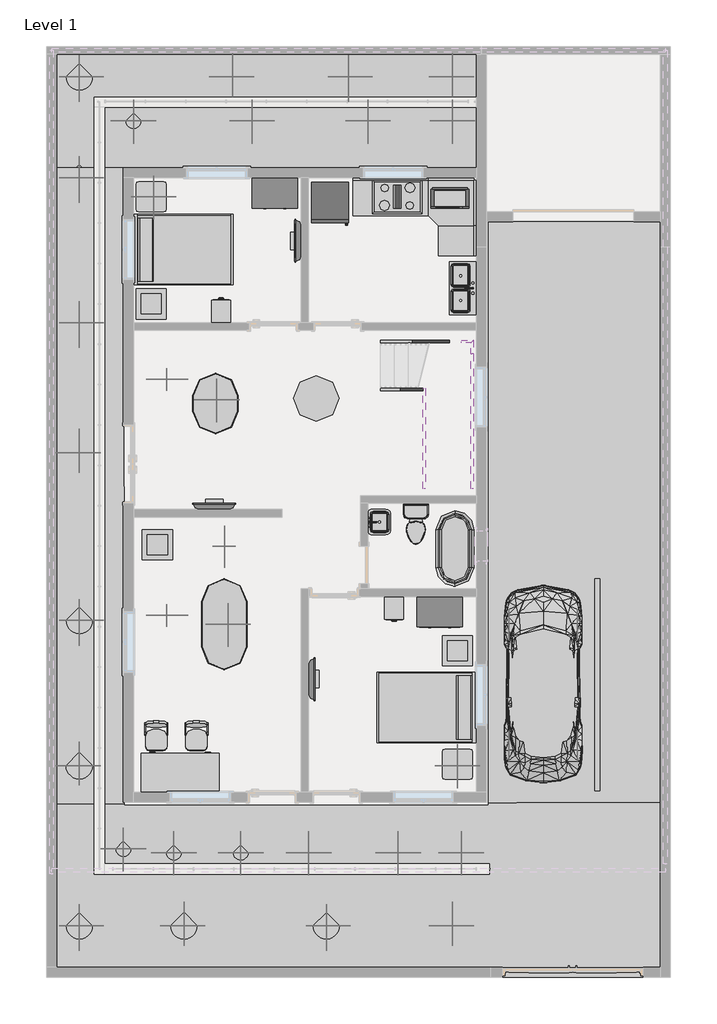
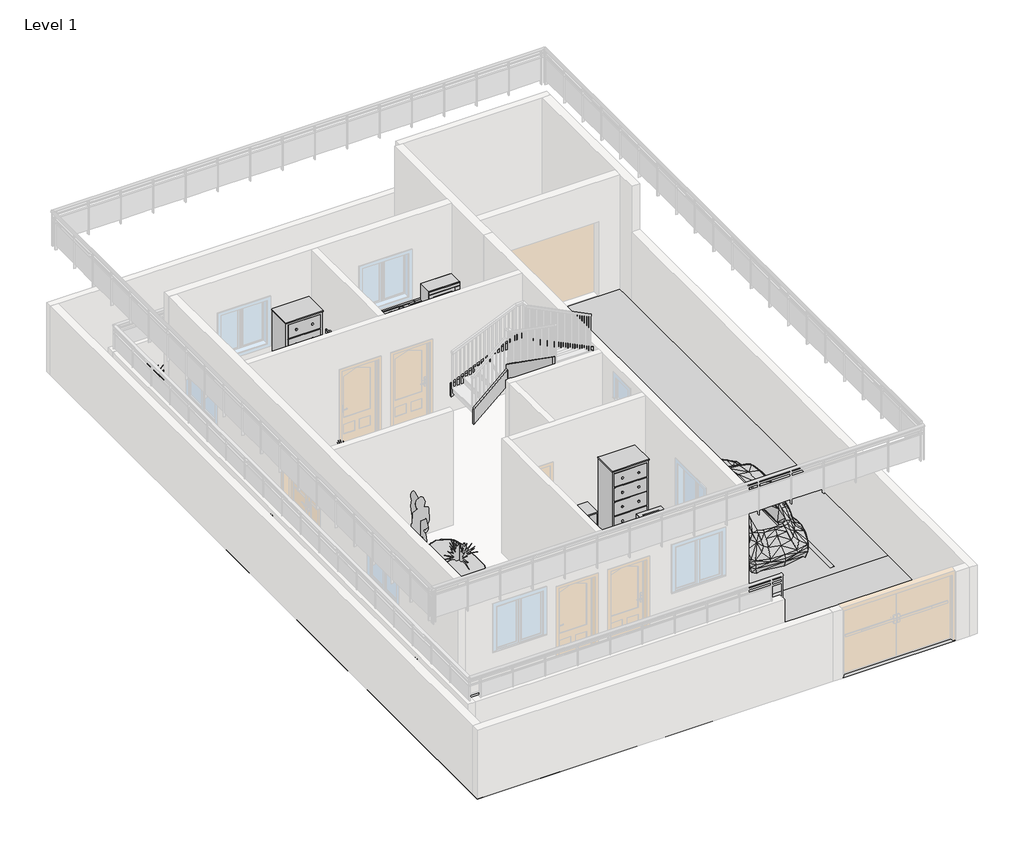
# One storey, part 5 of 5: 27 geographic elements, 21 furniture elements, 12 proxies, 6 members, 5 flow terminals.
"""IFC4 building model written with IfcOpenShell, lengths in millimetres."""

from ifc_helpers import new_model, si_unit, frame, origin, place, context, project, spatial, polyline, outline, extrude, triangles, transform, mapped, element, save
from components import proxy_bb1e6e30, proxy_8a8d5ab2, parking_space_9_x_18_90_deg_fdd9e8f5, rpc_beetle_rpc_beetle_3ce7ba48, rpc_female_69e001fa, proxy_a13a33b2, flow_terminal_accce45a, flow_terminal_a53be723, flow_terminal_62a433f7, toilet_domestic_3d_toilet_domestic_3d_f7549cf7, toilet_domestic_3d_toilet_domestic_3d_183bbd19, flow_terminal_b374fae2, furniture_096e7f55, furniture_bb55ed6b, furniture_072f6425, furniture_33655958, furniture_3d1d9cbc, furniture_56245f3a, furniture_b5c51a22, furniture_be1c6672, furniture_2c34a4f9, furniture_905aceb5, furniture_31d08a24, furniture_4f21b5ed, rpc_plant_tropical_55f6ff97, rpc_plant_tropical_agave_1_5_93a2a214, rpc_plant_tropical_jungle_flame_3_9c4808c2

model = new_model("IFC4")

# Units and contexts
model_context = context("Model", 3, world=origin())
ifc_project = project(units=[si_unit("LENGTHUNIT", "METRE", prefix="MILLI")], contexts=[model_context])

# Site, building, storey
site = spatial("IfcSite", under=ifc_project)
building = spatial("IfcBuilding", under=site)
storey = spatial("IfcBuildingStorey", under=building, Name="Level 1", Elevation=0.0)

# Proxies
placement = place(None, origin())
element("IfcBuildingElementProxy", 1, Name="Building Element Proxy", at=placement, inside=storey, context=model_context, shape_type="Tessellation", body=[
    triangles([(-2362.0350391, 11534.7029114, 0.0), (-2374.735136, 9147.103299, 0.0), (-2273.1350876, 9248.7034927, 0.0), (-11137.7352814, 9245.8391327, 0.0), (-11137.7352814, 11687.1029114, 0.0)], [[5, 4, 1], [2, 3, 1], [2, 1, 4]], closed=False),
])
element("IfcBuildingElementProxy", 2, Name="Building Element Proxy", at=placement, inside=storey, context=model_context, shape_type="Tessellation", body=[
    triangles([(-9588.3350876, 9248.7034927, 0.0), (-11137.7352814, 9247.2006775, 0.0), (-9588.3350876, -3527.4966042, 0.0), (-11137.7352814, -3577.79179, 0.0), (-9562.9348938, -3578.296701, 0.0)], [[2, 4, 3], [3, 5, 1], [5, 3, 4], [3, 1, 2]], closed=False),
])
element("IfcBuildingElementProxy", 3, Name="Building Element Proxy", at=placement, inside=storey, context=model_context, shape_type="Tessellation", body=[
    triangles([(-10934.5348938, -3567.3589966, 0.0), (-11137.7352814, -3577.79179, 0.0), (-11137.7352814, -7058.0965073, 0.0), (1435.264864, -7058.0965073, 0.0), (1435.264864, -3525.6286949, 0.0)], [[2, 3, 1], [1, 4, 5], [4, 1, 3]], closed=False),
])
element("IfcBuildingElementProxy", 4, Name="Building Element Proxy", at=placement, inside=storey, context=model_context, shape_type="Tessellation", body=[
    triangles([(-2273.1350876, -3527.4966042, 0.0), (1435.264864, -3483.8981026, 0.0), (-2273.1350876, 8156.503299, 0.0), (1232.0649124, 8156.503299, 0.0), (1232.0649124, -3528.5849098, 0.0), (-1984.8734676, -3532.3309021, 0.0), (-2247.7350391, -3578.296701, 0.0)], [[6, 3, 1], [6, 1, 7], [6, 5, 4], [5, 6, 7], [2, 4, 5], [6, 4, 3]], closed=False),
])
proxy_shape = proxy_bb1e6e30(model_context)
element("IfcBuildingElementProxy", 5, Name="Cook Top-4 Unit : 36\" x 20\"", ObjectType="Cook Top-4 Unit : 36\" x 20\"", at=placement, inside=storey, context=model_context, shape_type="MappedRepresentation", body=[
    mapped(proxy_shape, transform((-4070.1850785, 8664.5033005, 0.0), x_axis=(1.0, 0.0, 0.0), y_axis=(0.0, 1.0, 0.0), z_axis=(0.0, 0.0, 1.0))),
])
proxy_2_shape = proxy_8a8d5ab2(model_context)
element("IfcBuildingElementProxy", 6, Name="Microwave : 30\" x 16\" x 18\"", ObjectType="Microwave : 30\" x 16\" x 18\"", at=placement, inside=storey, context=model_context, shape_type="MappedRepresentation", body=[
    mapped(proxy_2_shape, transform((-3510.0279559, 8992.1838064, 0.0), x_axis=(1.0, 0.0, 0.0), y_axis=(0.0, 1.0, 0.0), z_axis=(0.0, 0.0, 1.0))),
])
parking_space_9_x_18_90_deg_shape = parking_space_9_x_18_90_deg_fdd9e8f5(model_context)
element("IfcBuildingElementProxy", 7, Name="Parking Space : 9' x 18' - 90 deg", ObjectType="Parking Space : 9' x 18' - 90 deg", at=placement, inside=storey, context=model_context, shape_type="MappedRepresentation", body=[
    mapped(parking_space_9_x_18_90_deg_shape, transform((-37.9350785, -3298.8966995, 0.0), x_axis=(-1.0000000000000004, 0.0, 0.0), y_axis=(0.0, -1.0000000000000004, 0.0), z_axis=(0.0, 0.0, 1.0))),
])
rpc_beetle_rpc_beetle_shape = rpc_beetle_rpc_beetle_3ce7ba48(model_context)
element("IfcBuildingElementProxy", 8, Name="RPC Beetle : RPC Beetle", ObjectType="RPC Beetle : RPC Beetle", at=placement, inside=storey, context=model_context, shape_type="MappedRepresentation", body=[
    mapped(rpc_beetle_rpc_beetle_shape, transform((-1130.1350785, -2384.4966995, 0.0), x_axis=(1.0, 0.0, 0.0), y_axis=(0.0, 1.0, 0.0), z_axis=(0.0, 0.0, 1.0))),
])
rpc_female_shape = rpc_female_69e001fa(model_context)
element("IfcBuildingElementProxy", 9, Name="RPC Female", ObjectType="RPC Female", at=placement, inside=storey, context=model_context, shape_type="MappedRepresentation", body=[
    mapped(rpc_female_shape, transform((-7557.9773474, 1463.6033005, 0.0), x_axis=(1.0, 0.0, 0.0), y_axis=(0.0, 1.0, 0.0), z_axis=(0.0, 0.0, 1.0))),
])
element("IfcBuildingElementProxy", 10, Name="RPC Female", ObjectType="RPC Female", at=placement, inside=storey, context=model_context, shape_type="MappedRepresentation", body=[
    mapped(rpc_female_shape, transform((-8559.6350785, 231.7033005, 0.0), x_axis=(0.0, 1.0, 0.0), y_axis=(-1.0, 0.0, 0.0), z_axis=(0.0, 0.0, 1.0))),
])
element("IfcBuildingElementProxy", 11, Name="RPC Female", ObjectType="RPC Female", at=placement, inside=storey, context=model_context, shape_type="MappedRepresentation", body=[
    mapped(rpc_female_shape, transform((-8559.6350785, 4981.5033005, 0.0), x_axis=(0.0, 1.0, 0.0), y_axis=(-1.0, 0.0, 0.0), z_axis=(0.0, 0.0, 1.0))),
])
proxy_3_shape = proxy_a13a33b2(model_context)
element("IfcBuildingElementProxy", 12, Name="Refrigerator : 30\" x 32\" RH", ObjectType="Refrigerator : 30\" x 32\" RH", at=placement, inside=storey, context=model_context, shape_type="MappedRepresentation", body=[
    mapped(proxy_3_shape, transform((-5427.4975785, 8561.704329, 0.0), x_axis=(1.0, 0.0, 0.0), y_axis=(0.0, 1.0, 0.0), z_axis=(0.0, 0.0, 1.0))),
])

# Flow terminals
flow_terminal_shape = flow_terminal_accce45a(model_context)
element("IfcFlowTerminal", 13, ObjectType="Floor Drain - Round : 5\" Strainer - 2\" Drain", at=placement, inside=storey, context=model_context, shape_type="MappedRepresentation", body=[
    mapped(flow_terminal_shape, transform((-3492.3350785, 942.9033005, 0.0), x_axis=(1.0, 0.0, 0.0), y_axis=(0.0, 1.0, 0.0), z_axis=(0.0, 0.0, 1.0))),
])
flow_terminal_2_shape = flow_terminal_a53be723(model_context)
element("IfcFlowTerminal", 14, ObjectType="Sink Kitchen-Double : 42\" x 21\"", at=placement, inside=storey, context=model_context, shape_type="MappedRepresentation", body=[
    mapped(flow_terminal_2_shape, transform((-2758.0804796, 6838.6925411, 0.0), x_axis=(0.0, -1.0000000000000004, 0.0), y_axis=(1.0000000000000004, 0.0, 0.0), z_axis=(0.0, 0.0, 1.0))),
])
flow_terminal_3_shape = flow_terminal_62a433f7(model_context)
element("IfcFlowTerminal", 15, ObjectType="Sink Vanity-Square : 20\" x 18\"", at=placement, inside=storey, context=model_context, shape_type="MappedRepresentation", body=[
    mapped(flow_terminal_3_shape, transform((-4480.5896774, 2095.61406, 0.0), x_axis=(0.0, 1.0000000000000002, 0.0), y_axis=(-1.0000000000000002, 0.0, 0.0), z_axis=(0.0, 0.0, 1.0))),
])
toilet_domestic_3d_toilet_domestic_3d_shape = toilet_domestic_3d_toilet_domestic_3d_f7549cf7(model_context)
toilet_domestic_3d_toilet_domestic_3d_2_shape = toilet_domestic_3d_toilet_domestic_3d_183bbd19(model_context)
element("IfcFlowTerminal", 16, ObjectType="Toilet-Domestic-3D : Toilet-Domestic-3D", at=placement, inside=storey, context=model_context, shape_type="MappedRepresentation", body=[
    mapped(toilet_domestic_3d_toilet_domestic_3d_shape, transform((-3695.5350785, 1972.2072732, 0.0), x_axis=(1.0, 0.0, 0.0), y_axis=(0.0, 1.0, 0.0), z_axis=(0.0, 0.0, 1.0))),
    mapped(toilet_domestic_3d_toilet_domestic_3d_2_shape, transform((-3695.5350785, 1972.2072732, 0.0), x_axis=(1.0, 0.0, 0.0), y_axis=(0.0, 1.0, 0.0), z_axis=(0.0, 0.0, 1.0))),
])
flow_terminal_4_shape = flow_terminal_b374fae2(model_context)
element("IfcFlowTerminal", 17, ObjectType="Tub-Free Standing-3D : 30\" x 60\"", at=placement, inside=storey, context=model_context, shape_type="MappedRepresentation", body=[
    mapped(flow_terminal_4_shape, transform((-2908.1350785, 1577.9033005, 0.0), x_axis=(1.0, 0.0, 0.0), y_axis=(0.0, 1.0, 0.0), z_axis=(0.0, 0.0, 1.0))),
])

# Furniture
furniture_shape = furniture_096e7f55(model_context)
element("IfcFurniture", 18, ObjectType="Bed-Shaker : Double 56\" x 78\"", at=placement, inside=storey, context=model_context, shape_type="MappedRepresentation", body=[
    mapped(furniture_shape, transform((-9359.7350785, 7616.7533005, 0.0), x_axis=(0.0, 1.0000000000000002, 0.0), y_axis=(-1.0000000000000002, 0.0, 0.0), z_axis=(0.0, 0.0, 1.0))),
])
element("IfcFurniture", 19, ObjectType="Bed-Shaker : Double 56\" x 78\"", at=placement, inside=storey, context=model_context, shape_type="MappedRepresentation", body=[
    mapped(furniture_shape, transform((-2501.7350785, -1641.5466995, 0.0), x_axis=(0.0, -1.0000000000000002, 0.0), y_axis=(1.0000000000000002, 0.0, 0.0), z_axis=(0.0, 0.0, 1.0))),
])
furniture_2_shape = furniture_bb55ed6b(model_context)
element("IfcFurniture", 20, ObjectType="Cabinet-File 2 Drawer : 15\" x 18\"", at=placement, inside=storey, context=model_context, shape_type="MappedRepresentation", body=[
    mapped(furniture_2_shape, transform((-7747.7315256, 6210.9690004, 0.0), x_axis=(-1.0, 0.0, 0.0), y_axis=(0.0, -1.0, 0.0), z_axis=(0.0, 0.0, 1.0))),
])
element("IfcFurniture", 21, ObjectType="Cabinet-File 2 Drawer : 15\" x 18\"", at=placement, inside=storey, context=model_context, shape_type="MappedRepresentation", body=[
    mapped(furniture_2_shape, transform((-4004.9552228, 526.2376007, 0.0), x_axis=(1.0, 0.0, 0.0), y_axis=(0.0, 1.0, 0.0), z_axis=(0.0, 0.0, 1.0))),
])
furniture_3_shape = furniture_072f6425(model_context)
element("IfcFurniture", 22, ObjectType="Desk : 60\" x 30\" Student", at=placement, inside=storey, context=model_context, shape_type="MappedRepresentation", body=[
    mapped(furniture_3_shape, transform((-9207.3350785, -3324.2966995, 0.0), x_axis=(1.0, 0.0, 0.0), y_axis=(0.0, 1.0, 0.0), z_axis=(0.0, 0.0, 1.0))),
])
furniture_4_shape = furniture_33655958(model_context)
element("IfcFurniture", 23, ObjectType="Dresser : 48\" x 72\" x 24\"", at=placement, inside=storey, context=model_context, shape_type="MappedRepresentation", body=[
    mapped(furniture_4_shape, transform((-6271.1418187, 9103.8662546, 0.0), x_axis=(1.0, 0.0, 0.0), y_axis=(0.0, 1.0, 0.0), z_axis=(0.0, 0.0, 1.0))),
])
element("IfcFurniture", 24, ObjectType="Dresser : 48\" x 72\" x 24\"", at=placement, inside=storey, context=model_context, shape_type="MappedRepresentation", body=[
    mapped(furniture_4_shape, transform((-2943.7418187, 671.0662546, 0.0), x_axis=(1.0, 0.0, 0.0), y_axis=(0.0, 1.0, 0.0), z_axis=(0.0, 0.0, 1.0))),
])
furniture_5_shape = furniture_3d1d9cbc(model_context)
element("IfcFurniture", 25, ObjectType="Seating-Auditorium : 18\" x 24\" x 30\"", at=placement, inside=storey, context=model_context, shape_type="MappedRepresentation", body=[
    mapped(furniture_5_shape, transform((-8767.2072097, -1991.4212896, 0.0), x_axis=(-1.0000000000000004, 0.0, 0.0), y_axis=(0.0, -1.0000000000000004, 0.0), z_axis=(0.0, 0.0, 1.0))),
])
element("IfcFurniture", 26, ObjectType="Seating-Auditorium : 18\" x 24\" x 30\"", at=placement, inside=storey, context=model_context, shape_type="MappedRepresentation", body=[
    mapped(furniture_5_shape, transform((-7954.4072097, -1991.4212896, 0.0), x_axis=(-1.0, 0.0, 0.0), y_axis=(0.0, -1.0, 0.0), z_axis=(0.0, 0.0, 1.0))),
])
furniture_6_shape = furniture_56245f3a(model_context)
element("IfcFurniture", 27, ObjectType="TV - Flat Screen : 32\"", at=placement, inside=storey, context=model_context, shape_type="MappedRepresentation", body=[
    mapped(furniture_6_shape, transform((-6065.4737022, 7771.5587864, 914.4), x_axis=(0.0, -1.0000000000000004, 0.0), y_axis=(1.0000000000000004, 0.0, 0.0), z_axis=(0.0, 0.0, 1.0))),
])
element("IfcFurniture", 28, ObjectType="TV - Flat Screen : 32\"", at=placement, inside=storey, context=model_context, shape_type="MappedRepresentation", body=[
    mapped(furniture_6_shape, transform((-7763.4795927, 2423.8419242, 1041.4), x_axis=(-1.0, 0.0, 0.0), y_axis=(0.0, -1.0, 0.0), z_axis=(0.0, 0.0, 1.0))),
])
element("IfcFurniture", 29, ObjectType="TV - Flat Screen : 32\"", at=placement, inside=storey, context=model_context, shape_type="MappedRepresentation", body=[
    mapped(furniture_6_shape, transform((-5795.9964549, -1047.0521853, 1041.4), x_axis=(0.0, 1.0000000000000002, 0.0), y_axis=(-1.0000000000000002, 0.0, 0.0), z_axis=(0.0, 0.0, 1.0))),
])
furniture_7_shape = furniture_b5c51a22(model_context)
element("IfcFurniture", 30, ObjectType="Table-Coffee : 24\" x 24\" x 24\"", at=placement, inside=storey, context=model_context, shape_type="MappedRepresentation", body=[
    mapped(furniture_7_shape, transform((-9047.8008452, 6410.2922227, 0.0), x_axis=(1.0, 0.0, 0.0), y_axis=(0.0, 1.0, 0.0), z_axis=(0.0, 0.0, 1.0))),
])
element("IfcFurniture", 31, ObjectType="Table-Coffee : 24\" x 24\" x 24\"", at=placement, inside=storey, context=model_context, shape_type="MappedRepresentation", body=[
    mapped(furniture_7_shape, transform((-2875.6008452, -574.7077773, 0.0), x_axis=(1.0, 0.0, 0.0), y_axis=(0.0, 1.0, 0.0), z_axis=(0.0, 0.0, 1.0))),
])
element("IfcFurniture", 32, ObjectType="Table-Coffee : 24\" x 24\" x 24\"", at=placement, inside=storey, context=model_context, shape_type="MappedRepresentation", body=[
    mapped(furniture_7_shape, transform((-8920.8008452, 1558.8922227, 0.0), x_axis=(1.0, 0.0, 0.0), y_axis=(0.0, 1.0, 0.0), z_axis=(0.0, 0.0, 1.0))),
])
furniture_8_shape = furniture_be1c6672(model_context)
element("IfcFurniture", 33, ObjectType="Table-Dining Oval : 36\" x 48\"", at=placement, inside=storey, context=model_context, shape_type="MappedRepresentation", body=[
    mapped(furniture_8_shape, transform((-8092.2334392, 4900.7229727, 0.0), x_axis=(0.0, 1.0000000000000002, 0.0), y_axis=(-1.0000000000000002, 0.0, 0.0), z_axis=(0.0, 0.0, 1.0))),
])
furniture_9_shape = furniture_2c34a4f9(model_context)
element("IfcFurniture", 34, ObjectType="Table-Dining Oval : 36\" x 72\"", at=placement, inside=storey, context=model_context, shape_type="MappedRepresentation", body=[
    mapped(furniture_9_shape, transform((-7914.4334392, 455.7229727, 0.0), x_axis=(0.0, 1.0, 0.0), y_axis=(-1.0, 0.0, 0.0), z_axis=(0.0, 0.0, 1.0))),
])
furniture_10_shape = furniture_905aceb5(model_context)
element("IfcFurniture", 35, ObjectType="Table-Dining Round w Chairs : 36\" Diameter", at=placement, inside=storey, context=model_context, shape_type="MappedRepresentation", body=[
    mapped(furniture_10_shape, transform((-5805.8170457, 4785.3819891, 0.0), x_axis=(1.0, 0.0, 0.0), y_axis=(0.0, 1.0, 0.0), z_axis=(0.0, 0.0, 1.0))),
])
furniture_11_shape = furniture_31d08a24(model_context)
element("IfcFurniture", 36, ObjectType="Table-End : 24\" x 24\"", at=placement, inside=storey, context=model_context, shape_type="MappedRepresentation", body=[
    mapped(furniture_11_shape, transform((-9338.0687088, 8512.1033005, 0.0), x_axis=(1.0, 0.0, 0.0), y_axis=(0.0, 1.0, 0.0), z_axis=(0.0, 0.0, 1.0))),
])
element("IfcFurniture", 37, ObjectType="Table-End : 24\" x 24\"", at=placement, inside=storey, context=model_context, shape_type="MappedRepresentation", body=[
    mapped(furniture_11_shape, transform((-3165.8687088, -2917.8966995, 0.0), x_axis=(1.0, 0.0, 0.0), y_axis=(0.0, 1.0, 0.0), z_axis=(0.0, 0.0, 1.0))),
])
furniture_12_shape = furniture_4f21b5ed(model_context)
element("IfcFurniture", 38, ObjectType="Work Station Cubicle : 96\" x 96\"", at=placement, inside=storey, context=model_context, shape_type="MappedRepresentation", body=[
    mapped(furniture_12_shape, transform((-1981.3120709, 8913.7715483, 0.0), x_axis=(0.0, -0.9999999999999998, 0.0), y_axis=(0.9999999999999998, 0.0, 0.0), z_axis=(0.0, 0.0, 1.0))),
])

# Geographic elements
rpc_plant_tropical_shape = rpc_plant_tropical_55f6ff97(model_context)
element("IfcGeographicElement", 39, ObjectType="RPC Plant - Tropical", at=placement, inside=storey, context=model_context, shape_type="MappedRepresentation", body=[
    mapped(rpc_plant_tropical_shape, transform((-5054.4350785, 11077.5033005, 0.0), x_axis=(1.0, 0.0, 0.0), y_axis=(0.0, 1.0, 0.0), z_axis=(0.0, 0.0, 1.0))),
])
element("IfcGeographicElement", 40, ObjectType="RPC Plant - Tropical", at=placement, inside=storey, context=model_context, shape_type="MappedRepresentation", body=[
    mapped(rpc_plant_tropical_shape, transform((-10477.3350785, 11077.5033005, 0.0), x_axis=(1.0, 0.0, 0.0), y_axis=(0.0, 1.0, 0.0), z_axis=(0.0, 0.0, 1.0))),
])
element("IfcGeographicElement", 41, ObjectType="RPC Plant - Tropical", at=placement, inside=storey, context=model_context, shape_type="MappedRepresentation", body=[
    mapped(rpc_plant_tropical_shape, transform((-10477.3350785, 9045.5033005, 0.0), x_axis=(1.0, 0.0, 0.0), y_axis=(0.0, 1.0, 0.0), z_axis=(0.0, 0.0, 1.0))),
])
element("IfcGeographicElement", 42, ObjectType="RPC Plant - Tropical", at=placement, inside=storey, context=model_context, shape_type="MappedRepresentation", body=[
    mapped(rpc_plant_tropical_shape, transform((-10477.3350785, 6124.5033005, 0.0), x_axis=(1.0, 0.0, 0.0), y_axis=(0.0, 1.0, 0.0), z_axis=(0.0, 0.0, 1.0))),
])
element("IfcGeographicElement", 43, ObjectType="RPC Plant - Tropical", at=placement, inside=storey, context=model_context, shape_type="MappedRepresentation", body=[
    mapped(rpc_plant_tropical_shape, transform((-10477.3350785, 130.1033005, 0.0), x_axis=(1.0, 0.0, 0.0), y_axis=(0.0, 1.0, 0.0), z_axis=(0.0, 0.0, 1.0))),
])
element("IfcGeographicElement", 44, ObjectType="RPC Plant - Tropical", at=placement, inside=storey, context=model_context, shape_type="MappedRepresentation", body=[
    mapped(rpc_plant_tropical_shape, transform((-10477.3350785, -6016.6966995, 0.0), x_axis=(1.0, 0.0, 0.0), y_axis=(0.0, 1.0, 0.0), z_axis=(0.0, 0.0, 1.0))),
])
element("IfcGeographicElement", 45, ObjectType="RPC Plant - Tropical", at=placement, inside=storey, context=model_context, shape_type="MappedRepresentation", body=[
    mapped(rpc_plant_tropical_shape, transform((-5498.9350785, -6016.6966995, 0.0), x_axis=(1.0, 0.0, 0.0), y_axis=(0.0, 1.0, 0.0), z_axis=(0.0, 0.0, 1.0))),
])
rpc_plant_tropical_agave_1_5_shape = rpc_plant_tropical_agave_1_5_93a2a214(model_context)
element("IfcGeographicElement", 46, ObjectType="RPC Plant - Tropical : Agave - 1.5'", at=placement, inside=storey, context=model_context, shape_type="MappedRepresentation", body=[
    mapped(rpc_plant_tropical_agave_1_5_shape, transform((-2958.9350785, 10188.5033005, 0.0), x_axis=(1.0, 0.0, 0.0), y_axis=(0.0, 1.0, 0.0), z_axis=(0.0, 0.0, 1.0))),
])
element("IfcGeographicElement", 47, ObjectType="RPC Plant - Tropical : Agave - 1.5'", at=placement, inside=storey, context=model_context, shape_type="MappedRepresentation", body=[
    mapped(rpc_plant_tropical_agave_1_5_shape, transform((-4660.7350785, 10188.5033005, 0.0), x_axis=(1.0, 0.0, 0.0), y_axis=(0.0, 1.0, 0.0), z_axis=(0.0, 0.0, 1.0))),
])
element("IfcGeographicElement", 48, ObjectType="RPC Plant - Tropical : Agave - 1.5'", at=placement, inside=storey, context=model_context, shape_type="MappedRepresentation", body=[
    mapped(rpc_plant_tropical_agave_1_5_shape, transform((-6997.5350785, 10188.5033005, 0.0), x_axis=(1.0, 0.0, 0.0), y_axis=(0.0, 1.0, 0.0), z_axis=(0.0, 0.0, 1.0))),
])
element("IfcGeographicElement", 49, ObjectType="RPC Plant - Tropical : Agave - 1.5'", at=placement, inside=storey, context=model_context, shape_type="MappedRepresentation", body=[
    mapped(rpc_plant_tropical_agave_1_5_shape, transform((-9385.1350785, 10188.5033005, 0.0), x_axis=(1.0, 0.0, 0.0), y_axis=(0.0, 1.0, 0.0), z_axis=(0.0, 0.0, 1.0))),
])
element("IfcGeographicElement", 50, ObjectType="RPC Plant - Tropical : Agave - 1.5'", at=placement, inside=storey, context=model_context, shape_type="MappedRepresentation", body=[
    mapped(rpc_plant_tropical_agave_1_5_shape, transform((-2781.1350785, -4543.4966995, 0.0), x_axis=(1.0, 0.0, 0.0), y_axis=(0.0, 1.0, 0.0), z_axis=(0.0, 0.0, 1.0))),
])
element("IfcGeographicElement", 51, ObjectType="RPC Plant - Tropical : Agave - 1.5'", at=placement, inside=storey, context=model_context, shape_type="MappedRepresentation", body=[
    mapped(rpc_plant_tropical_agave_1_5_shape, transform((-9588.3350785, -4467.2966995, 0.0), x_axis=(1.0, 0.0, 0.0), y_axis=(0.0, 1.0, 0.0), z_axis=(0.0, 0.0, 1.0))),
])
element("IfcGeographicElement", 52, ObjectType="RPC Plant - Tropical : Agave - 1.5'", at=placement, inside=storey, context=model_context, shape_type="MappedRepresentation", body=[
    mapped(rpc_plant_tropical_agave_1_5_shape, transform((-8572.3350785, -4543.4966995, 0.0), x_axis=(1.0, 0.0, 0.0), y_axis=(0.0, 1.0, 0.0), z_axis=(0.0, 0.0, 1.0))),
])
element("IfcGeographicElement", 53, ObjectType="RPC Plant - Tropical : Agave - 1.5'", at=placement, inside=storey, context=model_context, shape_type="MappedRepresentation", body=[
    mapped(rpc_plant_tropical_agave_1_5_shape, transform((-7226.1350785, -4543.4966995, 0.0), x_axis=(1.0, 0.0, 0.0), y_axis=(0.0, 1.0, 0.0), z_axis=(0.0, 0.0, 1.0))),
])
element("IfcGeographicElement", 54, ObjectType="RPC Plant - Tropical : Agave - 1.5'", at=placement, inside=storey, context=model_context, shape_type="MappedRepresentation", body=[
    mapped(rpc_plant_tropical_agave_1_5_shape, transform((-5854.5350785, -4543.4966995, 0.0), x_axis=(1.0, 0.0, 0.0), y_axis=(0.0, 1.0, 0.0), z_axis=(0.0, 0.0, 1.0))),
])
element("IfcGeographicElement", 55, ObjectType="RPC Plant - Tropical : Agave - 1.5'", at=placement, inside=storey, context=model_context, shape_type="MappedRepresentation", body=[
    mapped(rpc_plant_tropical_agave_1_5_shape, transform((-4051.1350785, -4543.4966995, 0.0), x_axis=(1.0, 0.0, 0.0), y_axis=(0.0, 1.0, 0.0), z_axis=(0.0, 0.0, 1.0))),
])
element("IfcGeographicElement", 56, ObjectType="RPC Plant - Tropical : Agave - 1.5'", at=placement, inside=storey, context=model_context, shape_type="MappedRepresentation", body=[
    mapped(rpc_plant_tropical_agave_1_5_shape, transform((-8978.7350785, 8664.5033005, 609.6), x_axis=(1.0, 0.0, 0.0), y_axis=(0.0, 1.0, 0.0), z_axis=(0.0, 0.0, 1.0))),
])
element("IfcGeographicElement", 57, ObjectType="RPC Plant - Tropical : Agave - 1.5'", at=placement, inside=storey, context=model_context, shape_type="MappedRepresentation", body=[
    mapped(rpc_plant_tropical_agave_1_5_shape, transform((-7708.7350785, 4575.1033005, 736.6), x_axis=(1.0, 0.0, 0.0), y_axis=(0.0, 1.0, 0.0), z_axis=(0.0, 0.0, 1.0))),
])
element("IfcGeographicElement", 58, ObjectType="RPC Plant - Tropical : Agave - 1.5'", at=placement, inside=storey, context=model_context, shape_type="MappedRepresentation", body=[
    mapped(rpc_plant_tropical_agave_1_5_shape, transform((-2857.3350785, -2790.8966995, 609.6), x_axis=(1.0, 0.0, 0.0), y_axis=(0.0, 1.0, 0.0), z_axis=(0.0, 0.0, 1.0))),
])
element("IfcGeographicElement", 59, ObjectType="RPC Plant - Tropical : Agave - 1.5'", at=placement, inside=storey, context=model_context, shape_type="MappedRepresentation", body=[
    mapped(rpc_plant_tropical_agave_1_5_shape, transform((-7480.1350785, 53.9033005, 736.6), x_axis=(1.0, 0.0, 0.0), y_axis=(0.0, 1.0, 0.0), z_axis=(0.0, 0.0, 1.0))),
])
rpc_plant_tropical_jungle_flame_3_shape = rpc_plant_tropical_jungle_flame_3_9c4808c2(model_context)
element("IfcGeographicElement", 60, ObjectType="RPC Plant - Tropical : Jungle Flame - 3'", at=placement, inside=storey, context=model_context, shape_type="MappedRepresentation", body=[
    mapped(rpc_plant_tropical_jungle_flame_3_shape, transform((-2958.9350785, 11077.5033005, 0.0), x_axis=(1.0, 0.0, 0.0), y_axis=(0.0, 1.0, 0.0), z_axis=(0.0, 0.0, 1.0))),
])
element("IfcGeographicElement", 61, ObjectType="RPC Plant - Tropical : Jungle Flame - 3'", at=placement, inside=storey, context=model_context, shape_type="MappedRepresentation", body=[
    mapped(rpc_plant_tropical_jungle_flame_3_shape, transform((-7391.2350785, 11077.5033005, 0.0), x_axis=(1.0, 0.0, 0.0), y_axis=(0.0, 1.0, 0.0), z_axis=(0.0, 0.0, 1.0))),
])
element("IfcGeographicElement", 62, ObjectType="RPC Plant - Tropical : Jungle Flame - 3'", at=placement, inside=storey, context=model_context, shape_type="MappedRepresentation", body=[
    mapped(rpc_plant_tropical_jungle_flame_3_shape, transform((-10477.3350785, 3508.3033005, 0.0), x_axis=(1.0, 0.0, 0.0), y_axis=(0.0, 1.0, 0.0), z_axis=(0.0, 0.0, 1.0))),
])
element("IfcGeographicElement", 63, ObjectType="RPC Plant - Tropical : Jungle Flame - 3'", at=placement, inside=storey, context=model_context, shape_type="MappedRepresentation", body=[
    mapped(rpc_plant_tropical_jungle_flame_3_shape, transform((-10477.3350785, -2790.8966995, 0.0), x_axis=(1.0, 0.0, 0.0), y_axis=(0.0, 1.0, 0.0), z_axis=(0.0, 0.0, 1.0))),
])
element("IfcGeographicElement", 64, ObjectType="RPC Plant - Tropical : Jungle Flame - 3'", at=placement, inside=storey, context=model_context, shape_type="MappedRepresentation", body=[
    mapped(rpc_plant_tropical_jungle_flame_3_shape, transform((-8369.1350785, -6016.6966995, 0.0), x_axis=(1.0, 0.0, 0.0), y_axis=(0.0, 1.0, 0.0), z_axis=(0.0, 0.0, 1.0))),
])
element("IfcGeographicElement", 65, ObjectType="RPC Plant - Tropical : Jungle Flame - 3'", at=placement, inside=storey, context=model_context, shape_type="MappedRepresentation", body=[
    mapped(rpc_plant_tropical_jungle_flame_3_shape, transform((-2958.9350785, -6016.6966995, 0.0), x_axis=(1.0, 0.0, 0.0), y_axis=(0.0, 1.0, 0.0), z_axis=(0.0, 0.0, 1.0))),
])

# Members
element("IfcMember", 66, ObjectType="Stringer - 2\" Width", at=placement, inside=storey, context=model_context, shape_type="SweptSolid", body=[
    extrude(outline(polyline([(922.8849999, -4406.7350785), (590.0562463, -4406.7350785), (1305.2683876, -2776.0728858), (1638.0971411, -2776.0728858), (922.8849999, -4406.7350785)])), frame((0.0, 5718.1033005, 0.0), z_axis=(0.0, 1.0, 0.0), x_axis=(0.0, 0.0, 1.0)), (0.0, 0.0, 1.0), 50.8),
])
element("IfcMember", 67, ObjectType="Stringer - 2\" Width", at=placement, inside=storey, context=model_context, shape_type="SweptSolid", body=[
    extrude(outline(polyline([(-2776.0728858, 5718.1033005), (-2776.0728858, 5768.9033005), (-2537.598089, 5768.9033005), (-2588.398089, 5718.1033005), (-2776.0728858, 5718.1033005)])), frame((0.0, 0.0, 1305.2683876), z_axis=(0.0, 0.0, 1.0), x_axis=(1.0, 0.0, 0.0)), (0.0, 0.0, 1.0), 332.8287535),
])
element("IfcMember", 68, ObjectType="Stringer - 2\" Width", at=placement, inside=storey, context=model_context, shape_type="SweptSolid", body=[
    extrude(outline(polyline([(-2588.398089, 5718.1033005), (-2537.598089, 5768.9033005), (-2537.598089, 5499.9499575), (-2588.398089, 5499.9499575), (-2588.398089, 5718.1033005)])), frame((0.0, 0.0, 1305.2683876), z_axis=(0.0, 0.0, 1.0), x_axis=(1.0, 0.0, 0.0)), (0.0, 0.0, 1.0), 332.8287535),
])
element("IfcMember", 69, ObjectType="Stringer - 2\" Width", at=placement, inside=storey, context=model_context, shape_type="SweptSolid", body=[
    extrude(outline(polyline([(5499.9499575, 1638.0971411), (5499.9499575, 1305.2683876), (2782.166311, 2720.7901969), (2782.166311, 3053.6189504), (5499.9499575, 1638.0971411)])), frame((-2588.398089, 0.0, 0.0), z_axis=(1.0, 0.0, 0.0), x_axis=(0.0, 1.0, 0.0)), (0.0, 0.0, 1.0), 50.8),
])
element("IfcMember", 70, ObjectType="Stringer - 2\" Width", at=placement, inside=storey, context=model_context, shape_type="SweptSolid", body=[
    extrude(outline(polyline([(842.634734, -4406.7350785), (435.4922729, -4406.7350785), (1191.0265733, -3553.598089), (1598.1690344, -3553.598089), (842.634734, -4406.7350785)])), frame((0.0, 4752.9033005, 0.0), z_axis=(0.0, 1.0, 0.0), x_axis=(0.0, 0.0, 1.0)), (0.0, 0.0, 1.0), 50.8),
])
element("IfcMember", 71, ObjectType="Stringer - 2\" Width", at=placement, inside=storey, context=model_context, shape_type="SweptSolid", body=[
    extrude(outline(polyline([(4803.7033005, 1709.9296678), (4803.7033005, 1337.7212805), (2782.166311, 2754.5609981), (2782.166311, 3126.7693854), (4803.7033005, 1709.9296678)])), frame((-3553.598089, 0.0, 0.0), z_axis=(1.0, 0.0, 0.0), x_axis=(0.0, 1.0, 0.0)), (0.0, 0.0, 1.0), 50.8),
])

save(model, "model.ifc")

# Revit data of these elements
# Type "Cook Top-4 Unit : 36\" x 20\""
#   Assembly Code = "E1090400"
#   Depth = 2' - 0"
#   Width = 3' - 0"
#   Burner Material = Steel, Chrome Plated
#   Cooktop Material = Steel, Polished
#   Default Elevation = 0
# Type "Microwave : 30\" x 16\" x 18\""
#   Assembly Code = "E1090400"
#   Depth = 1' - 4"
#   Height = 1' - 6"
#   Width = 2' - 6"
#   Microwave Material = Laminate, Ivory, Matte
#   Default Elevation = 0
# Type "Parking Space : 9' x 18' - 90 deg"
#   Angle = 90.00°
#   Parking Length = 18' - 0"
#   Parking Width = 9' - 0"
#   pl = 14' - 0"
#   pw = 7' - 0"
# Type "RPC Beetle : RPC Beetle"
#   built-in parameter 1005195 = "RPC-16-0U6E-L4EG-ENH1-J3KF-SVEL-0TX4-C0"
#   Height = 0
# Type "RPC Female"
#   built-in parameter 1005195 = "RPC-8-FXA2-QQQ0-UGV2-6"
#   Height = 0
# Type "Refrigerator : 30\" x 32\" RH"
#   Label = "REF."
#   Assembly Code = "E1090400"
#   Depth = 2' - 7 3/4"
#   Handle = 2' - 3"
#   Height = 5' - 10"
#   Rear Clearance = 0' - 2"
#   Top Door Height = 1' - 8"
#   Width = 2' - 5 3/8"
#   Material = Carpet (1)
#   Default Elevation = 0
# Type "Floor Drain - Round : 5\" Strainer - 2\" Drain"
#   WFU = 2
#   Strainer Height = 0' - 3 1/4"
#   Strainer Radius = 0' - 2 1/2"
#   Strainer Diameter = 0' - 5"
#   Radius 6 = 0' - 0 5/8"
#   Radius 5 = 0' - 1 1/4"
#   Radius 4 = 0' - 1 7/8"
#   Radius 2 = 0' - 3.04167"
#   Radius 1 = 0' - 2.02083"
#   Radius 3 = 0' - 2 1/32"
#   Pipe Radius = 1"
#   Pipe Diameter = 2"
#   Height 2 = 0' - 0.725"
#   Height 1 = 0' - 1 13/16"
#   Body Radius = 0' - 4 1/16"
#   Body Height = 0' - 3 5/8"
#   Body Diameter = 0' - 8 1/8"
#   Drain Material = none
#   HWFU = 0
#   Default Elevation = 0
#   CWFU = 0
# Type "Sink Kitchen-Double : 42\" x 21\""
#   Assembly Code = "D2010410"
#   Counter Height = 3' - 0"
#   Depth = 1' - 9"
#   Width = 3' - 6"
#   Faucet Material = Steel, Polished
#   Sink Material = Steel, Polished
#   Default Elevation = 0
# Type "Sink Vanity-Square : 20\" x 18\""
#   Assembly Code = "D2010400"
#   Counter Height = 2' - 7"
#   Depth = 1' - 6"
#   Width = 1' - 8"
#   Basin Material = Porcelain, Linen
#   Faucet Material = Steel, Polished
#   Default Elevation = 0
# Type "Toilet-Domestic-3D : Toilet-Domestic-3D"
#   Assembly Code = "D2010110"
#   Toilet - Bowl/Basin Material = Porcelain, Linen
#   Toilet - Seat Material = Laminate, Linen, Matte
#   Default Elevation = 0
# Type "Tub-Free Standing-3D : 30\" x 60\""
#   Assembly Code = "D2010110"
#   Height = 1' - 6"
#   Length = 5' - 0"
#   Width = 2' - 6"
#   Tub Material = Porcelain, Ivory
#   Default Elevation = 0
# Type "Bed-Shaker : Double 56\" x 78\""
#   Assembly Code = "E2020200"
#   Length = 6' - 6"
#   Width = 4' - 8"
#   Frame Material = Birch
#   Mattress Material = Plywood, Sheathing
#   Default Elevation = 0
# Type "Cabinet-File 2 Drawer : 15\" x 18\""
#   Assembly Code = "E2020200"
#   Depth = 1' - 6"
#   Height = 2' - 5"
#   Width = 1' - 3"
#   Cabinet Material = Steel, Paint Finish, Ivory, Glossy
#   Handle Material = Steel, Chrome Plated
#   Default Elevation = 0
# Type "Desk : 60\" x 30\" Student"
#   Assembly Code = "E2020200"
#   Depth = 2' - 6"
#   Height = 2' - 6"
#   Leg Height = 0' - 6"
#   Width = 5' - 0"
#   Body Material = Laminate, Ivory, Matte
#   Handle/Leg Material = Steel, Chrome Plated
#   Top Material = Cherry
#   Default Elevation = 0
# Type "Dresser : 48\" x 72\" x 24\""
#   Assembly Code = "E2020200"
#   Depth = 2' - 0"
#   Height = 6' - 0"
#   Width = 3' - 0"
#   Dresser Material = Wood - Teak
#   Drawer Material = Wood - Teak
#   Knob Material = Cherry
#   Default Elevation = 0
# Type "Seating-Auditorium : 18\" x 24\" x 30\""
#   Assembly Code = "E2020200"
#   Seat Material = Linen, Beige
#   Frame Material = Steel, Paint Finish, Dark Gray, Matte
#   Default Elevation = 0
# Type "TV - Flat Screen : 32\""
#   SinAng = 0' - 0.0193"
#   L = 2' - 3.79372"
#   H = 1' - 3.6354"
#   Thickness = 0' - 4.33071"
#   Diagonal = 2' - 7.88976"
#   CosAng = 0' - 0.03431"
#   Stand [instance default] = yes
#   Default Elevation = 0
# Type "Table-Coffee : 24\" x 24\" x 24\""
#   Assembly Code = "E2020200"
#   Height = 2' - 0"
#   Length = 2' - 0"
#   Width = 2' - 0"
#   Top Material = none
#   Frame Material = none
#   Default Elevation = 0
# Type "Table-Dining Oval : 36\" x 48\""
#   Assembly Code = "E2020200"
#   Length = 4' - 0"
#   Width = 3' - 0"
#   Base Material = Steel, Chrome Plated
#   Top Material = Glass - Clear, Grey
#   Default Elevation = 0
#   Description = (empty or 0)
# Type "Table-Dining Oval : 36\" x 72\""
#   Assembly Code = "E2020200"
#   Length = 6' - 0"
#   Width = 3' - 0"
#   Base Material = Steel, Chrome Plated
#   Top Material = Glass - Clear, Grey
#   Default Elevation = 0
#   Description = (empty or 0)
# Type "Table-Dining Round w Chairs : 36\" Diameter"
#   Assembly Code = "E2020200"
#   Radius = 1' - 6"
#   Diameter = 3' - 0"
#   Height = 2' - 6"
#   Chairs = 4
#   Base Material = Pine
#   Top Material = Laminate, Linen, Matte
#   Default Elevation = 0
# Type "Table-End : 24\" x 24\""
#   Assembly Code = "E2020200"
#   Height = 2' - 0"
#   Length = 2' - 0"
#   Width = 2' - 0"
#   Base Material = Birch
#   Top Material = Laminate, Ivory, Matte
#   Default Elevation = 0
# Type "Work Station Cubicle : 96\" x 96\""
#   Assembly Code = "E2020"
#   Desktop Height = 2' - 6"
#   Desktop1 Width = 2' - 4"
#   Desktop2 Width = 2' - 4"
#   Panel Height = 2' - 8"
#   Panel1 Length = 5' - 0"
#   Panel2 Length = 2' - 0"
#   Cube Panel Material = Textile - Light Gray
#   Work Top Material = Laminate, Ivory, Matte
#   Default Elevation = 0
# Type "RPC Plant - Tropical"
#   built-in parameter 1005198 = "{2, 15},{39, RPC-16-FWM5-GM7X-C67P-4000-ST1L-LVER-AU},{1, 0},{1, 0},{2, 13},{1, 8},{5, Color},{1, 0},{1, 0},{3, 0.8},{3, 0.8},{3, 0.8},{1, 8},{7, BBoxMin},{1, 0},{1, 0},{1, 0},{1, 0},{1, 0},{1, 8},{7, BBoxMax},{1, 0},{1, 0},{1, 0},{1, 0},{1, 0},{2, 11},{9, RPCTypeId},{1, 0},{1, 0},{39, RPC-16-FWM5-GM7X-C67P-4000-ST1L-LVER-AU},{1, 6},{14, RPCPlantHeight},{1, 0},{1, 0},{1, 3},{2, 11},{7, keyword},{1, 0},{1, 0},{35, :RPCs:Shrubs [General]:Geometry:RPC},{2, 11},{8, category},{1, 0},{1, 0},{16, Shrubs [General]},{2, 11},{12, LocalizedUID},{1, 0},{1, 0},{10, Crane Lily},{2, 14},{6, Height},{1, 0},{1, 0},{1, 3},{1, 2},{16, Cast Reflections},{1, 0},{1, 0},{1, 0},{1, 2},{12, Cast Shadows},{1, 0},{1, 0},{1, 1},{1, 2},{9, Lock View},{1, 0},{1, 0},{1, 0},{1, 4},{5, ViewC},{1, 0},{1, 0},{1, 0},{21, assetlibrary_base.fbx},{1, 5},"
#   built-in parameter 1005195 = "RPC-16-FWM5-GM7X-C67P-4000-ST1L-LVER-AU"
#   Assembly Code = "G2050500"
#   Height = 3' - 0"
#   Default Elevation = 0
# Type "RPC Plant - Tropical : Agave - 1.5'"
#   built-in parameter 1005198 = "{2, 15},{39, RPC-16-G1GJ-63FX-7K5P-N000-ST1L-LVER-AU},{1, 0},{1, 0},{2, 13},{1, 8},{5, Color},{1, 0},{1, 0},{3, 0.8},{3, 0.8},{3, 0.8},{1, 8},{7, BBoxMin},{1, 0},{1, 0},{1, 0},{1, 0},{1, 0},{1, 8},{7, BBoxMax},{1, 0},{1, 0},{1, 0},{1, 0},{1, 0},{2, 11},{9, RPCTypeId},{1, 0},{1, 0},{39, RPC-16-G1GJ-63FX-7K5P-N000-ST1L-LVER-AU},{1, 6},{14, RPCPlantHeight},{1, 0},{1, 0},{3, 1.5},{2, 11},{7, keyword},{1, 0},{1, 0},{35, :RPCs:Plants [General]:Geometry:RPC},{2, 11},{8, category},{1, 0},{1, 0},{16, Plants [General]},{2, 11},{12, LocalizedUID},{1, 0},{1, 0},{5, Agave},{2, 14},{6, Height},{1, 0},{1, 0},{3, 1.5},{1, 2},{16, Cast Reflections},{1, 0},{1, 0},{1, 0},{1, 2},{12, Cast Shadows},{1, 0},{1, 0},{1, 1},{1, 2},{9, Lock View},{1, 0},{1, 0},{1, 0},{1, 4},{5, ViewC},{1, 0},{1, 0},{1, 0},{21, assetlibrary_base.fbx},{1, 5},"
#   built-in parameter 1005195 = "RPC-16-G1GJ-63FX-7K5P-N000-ST1L-LVER-AU"
#   Type Comments = "Agave"
#   Assembly Code = "G2050500"
#   Height = 1' - 6"
#   Default Elevation = 0
# Type "RPC Plant - Tropical : Jungle Flame - 3'"
#   built-in parameter 1005198 = "{2, 15},{39, RPC-16-FUVJ-JWG0-MWGK-8000-ST1L-LVER-AU},{1, 0},{1, 0},{2, 13},{1, 8},{5, Color},{1, 0},{1, 0},{3, 0.8},{3, 0.8},{3, 0.8},{1, 8},{7, BBoxMin},{1, 0},{1, 0},{1, 0},{1, 0},{1, 0},{1, 8},{7, BBoxMax},{1, 0},{1, 0},{1, 0},{1, 0},{1, 0},{2, 11},{9, RPCTypeId},{1, 0},{1, 0},{39, RPC-16-FUVJ-JWG0-MWGK-8000-ST1L-LVER-AU},{1, 6},{14, RPCPlantHeight},{1, 0},{1, 0},{1, 3},{2, 11},{7, keyword},{1, 0},{1, 0},{35, :RPCs:Shrubs [General]:Geometry:RPC},{2, 11},{8, category},{1, 0},{1, 0},{16, Shrubs [General]},{2, 11},{12, LocalizedUID},{1, 0},{1, 0},{12, Jungle Flame},{2, 14},{6, Height},{1, 0},{1, 0},{1, 3},{1, 2},{16, Cast Reflections},{1, 0},{1, 0},{1, 0},{1, 2},{12, Cast Shadows},{1, 0},{1, 0},{1, 1},{1, 2},{9, Lock View},{1, 0},{1, 0},{1, 0},{1, 4},{5, ViewC},{1, 0},{1, 0},{1, 0},{21, assetlibrary_base.fbx},{1, 5},"
#   built-in parameter 1005195 = "RPC-16-FUVJ-JWG0-MWGK-8000-ST1L-LVER-AU"
#   Type Comments = "Jungle Flame"
#   Assembly Code = "G2050500"
#   Height = 3' - 0"
#   Default Elevation = 0
# Elements 1, 2, 3, 4 (IfcBuildingElementProxy)
#   Material = none
#   Phase Created = New Construction
# Element 5 (IfcBuildingElementProxy, "Cook Top-4 Unit : 36\" x 20\"")
#   Phase Created = New Construction
#   Materials on its faces: "Steel, Chrome Plated", "Steel, Polished"
# Element 6 (IfcBuildingElementProxy, "Microwave : 30\" x 16\" x 18\"")
#   Phase Created = New Construction
#   Materials on its faces: "Laminate, Ivory, Matte", "Glass"
# Element 7 (IfcBuildingElementProxy, "Parking Space : 9' x 18' - 90 deg")
#   Phase Created = New Construction
#   Materials on its faces: "Parking Stripe"
# Element 8 (IfcBuildingElementProxy, "RPC Beetle : RPC Beetle")
#   Phase Created = New Construction
# Elements 9, 10, 11 (IfcBuildingElementProxy, "RPC Female")
#   Phase Created = New Construction
# Element 12 (IfcBuildingElementProxy, "Refrigerator : 30\" x 32\" RH")
#   Phase Created = New Construction
#   Materials on its faces: "Carpet (1)", "Steel, Chrome Plated"
# Element 13 (IfcFlowTerminal, "Floor Drain - Round : 5\" Strainer - 2\" Drain")
#   Mark = "5"
#   Phase Created = New Construction
# Element 14 (IfcFlowTerminal, "Sink Kitchen-Double : 42\" x 21\"")
#   Mark = "1"
#   Phase Created = New Construction
#   Materials on its faces: "Steel, Polished"
# Element 15 (IfcFlowTerminal, "Sink Vanity-Square : 20\" x 18\"")
#   Mark = "2"
#   Phase Created = New Construction
#   Materials on its faces: "Porcelain, Linen", "Steel, Polished"
# Element 16 (IfcFlowTerminal, "Toilet-Domestic-3D : Toilet-Domestic-3D")
#   Mark = "3"
#   Phase Created = New Construction
#   Materials on its faces: "Porcelain, Linen", "Laminate, Linen, Matte"
# Element 17 (IfcFlowTerminal, "Tub-Free Standing-3D : 30\" x 60\"")
#   Mark = "4"
#   Phase Created = New Construction
#   Materials on its faces: "Porcelain, Ivory"
# Elements 18, 19 (IfcFurniture, "Bed-Shaker : Double 56\" x 78\"")
#   Phase Created = New Construction
#   Materials on its faces: "Birch", "Plywood, Sheathing"
# Elements 20, 21 (IfcFurniture, "Cabinet-File 2 Drawer : 15\" x 18\"")
#   Phase Created = New Construction
#   Materials on its faces: "Steel, Chrome Plated", "Steel, Paint Finish, Ivory, Glossy"
# Element 22 (IfcFurniture, "Desk : 60\" x 30\" Student")
#   Phase Created = New Construction
#   Materials on its faces: "Steel, Chrome Plated", "Laminate, Ivory, Matte", "Cherry"
# Elements 23, 24 (IfcFurniture, "Dresser : 48\" x 72\" x 24\"")
#   Phase Created = New Construction
#   Materials on its faces: "Laminate, Ivory, Matte", "Cherry", "Wood - Teak"
# Elements 25, 26 (IfcFurniture, "Seating-Auditorium : 18\" x 24\" x 30\"")
#   Phase Created = New Construction
#   Materials on its faces: "Steel, Paint Finish, Dark Gray, Matte", "Linen, Beige"
# Elements 27, 28, 29 (IfcFurniture, "TV - Flat Screen : 32\"")
#   Stand = yes
#   Phase Created = New Construction
#   Materials on its faces: "TV - Black", "TV - Glass", "TV - Screen"
# Elements 30, 31, 32 (IfcFurniture, "Table-Coffee : 24\" x 24\" x 24\"")
#   Phase Created = New Construction
#   Materials on its faces: "Glass - Clear, Grey"
# Element 33 (IfcFurniture, "Table-Dining Oval : 36\" x 48\"")
#   Phase Created = New Construction
#   Materials on its faces: "Steel, Chrome Plated", "Glass - Clear, Grey"
# Element 34 (IfcFurniture, "Table-Dining Oval : 36\" x 72\"")
#   Phase Created = New Construction
#   Materials on its faces: "Steel, Chrome Plated", "Glass - Clear, Grey"
# Element 35 (IfcFurniture, "Table-Dining Round w Chairs : 36\" Diameter")
#   Phase Created = New Construction
#   Materials on its faces: "Pine", "Laminate, Linen, Matte"
# Elements 36, 37 (IfcFurniture, "Table-End : 24\" x 24\"")
#   Phase Created = New Construction
#   Materials on its faces: "Laminate, Ivory, Matte", "Birch"
# Element 38 (IfcFurniture, "Work Station Cubicle : 96\" x 96\"")
#   Phase Created = New Construction
#   Materials on its faces: "Textile - Light Gray", "Laminate, Ivory, Matte"
# Elements 39, 40, 41, 42, 43, 44, 45 (IfcGeographicElement, "RPC Plant - Tropical")
#   Phase Created = New Construction
# Elements 46, 47, 48, 49, 50, 51, 52, 53, 54, 55, 56, 57, 58, 59 (IfcGeographicElement, "RPC Plant - Tropical : Agave - 1.5'")
#   Phase Created = New Construction
# Elements 60, 61, 62, 63, 64, 65 (IfcGeographicElement, "RPC Plant - Tropical : Jungle Flame - 3'")
#   Phase Created = New Construction
# Elements 66, 67, 68, 69, 70, 71 (IfcMember, "Stringer - 2\" Width")
#   Phase Created = New Construction
# Materials
#   "Steel, Chrome Plated": class "Metal", colour RGB 17 17 17, transparency 0, Description = "Chromiuim plated steel", Cost = 0
#   "Steel, Polished": class "Metal", colour RGB 57 57 57, transparency 0, Description = "Polished steel", Cost = 0
#   "Laminate, Ivory, Matte": class "Plastic", colour RGB 247 247 239, transparency 0, Description = "Plastic Laminate - Ivory, Matte", Cost = 0
#   "Carpet (1)": class "Carpet", colour RGB 124 80 67, transparency 0, Description = "Interior finish"
#   "Porcelain, Linen": class "Ceramic", colour RGB 249 239 230, transparency 0, Description = "Porcelain, linen", Cost = 0
#   "Laminate, Linen, Matte": class "Plastic", colour RGB 249 239 230, transparency 0, Description = "Plastic Laminate - Linen, Matte", Cost = 0
#   "Porcelain, Ivory": class "Ceramic", colour RGB 247 247 239, transparency 0, Description = "Porcelain, ivory", Cost = 0
#   "Birch": class "Wood", colour RGB 224 178 126, transparency 0, Description = "Betula Alleghaniensis", Cost = 0
#   "Plywood, Sheathing": class "Wood", colour RGB 212 179 113, transparency 0, Description = "Plywood, sheathing grade", Cost = 0
#   "Steel, Paint Finish, Ivory, Glossy": class "Metal", colour RGB 247 247 239, transparency 0, Description = "Steel, paint finish, ivory, glossy", Cost = 0
#   "Cherry": class "Wood", colour RGB 226 177 128, transparency 0, Description = "Prunus Serotina", Cost = 0
#   "Wood - Teak": class "Wood", colour RGB 145 112 90, transparency 0
#   "Linen, Beige": class "Textile", colour RGB 249 239 230, transparency 0, Description = "Linen, beige", Cost = 0
#   "Steel, Paint Finish, Dark Gray, Matte": class "Metal", colour RGB 0 0 0, transparency 0, Description = "Steel, paint finish, dark gray, matte", Cost = 0
#   "Glass - Clear, Grey": class "Glass", colour RGB 252 255 255, transparency 0.64
#   "Pine": class "Wood", colour RGB 223 192 134, transparency 0, Description = "Pinus Echinata", Cost = 0
#   "Textile - Light Gray": class "Fabric", colour RGB 204 204 204, transparency 0
#   "Glass": class "Glass", colour RGB 0 128 192, transparency 0.75, Description = "Soda Lime Glass", Cost = 0
#   "Parking Stripe": class "Paint", colour RGB 250 250 91, transparency 0
#   "TV - Black": colour RGB 49 49 49, transparency 0
#   "TV - Glass": colour RGB 157 157 157, transparency 0.9
#   "TV - Screen": colour RGB 0 0 0, transparency 0
